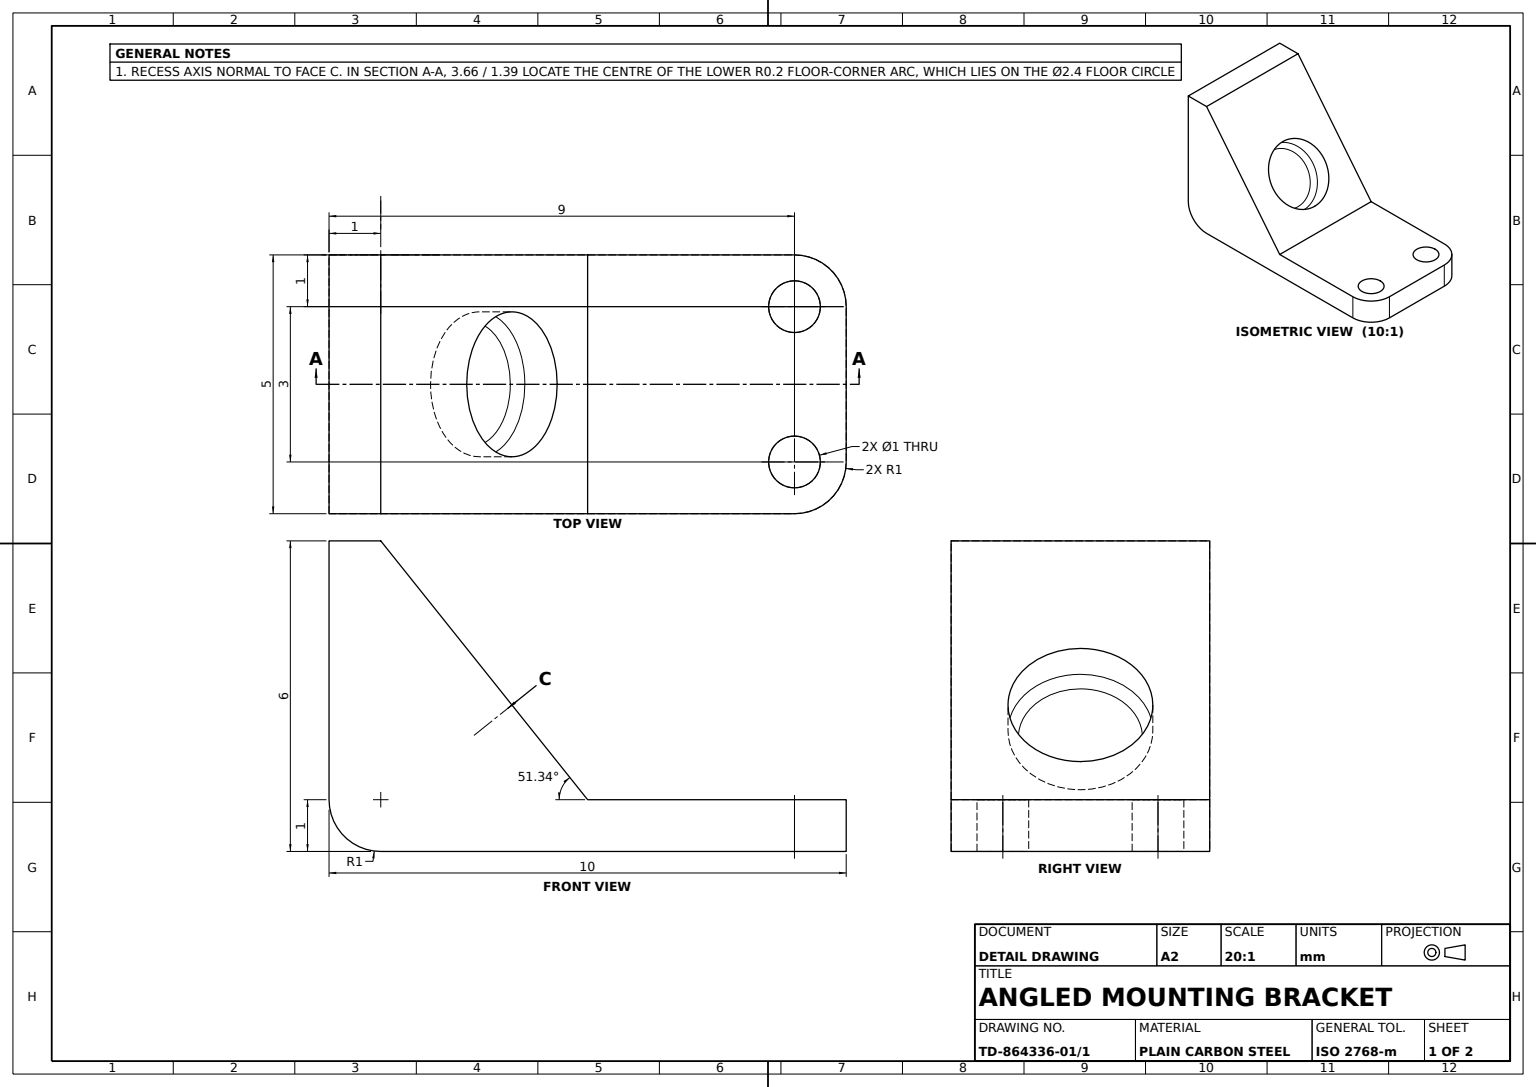
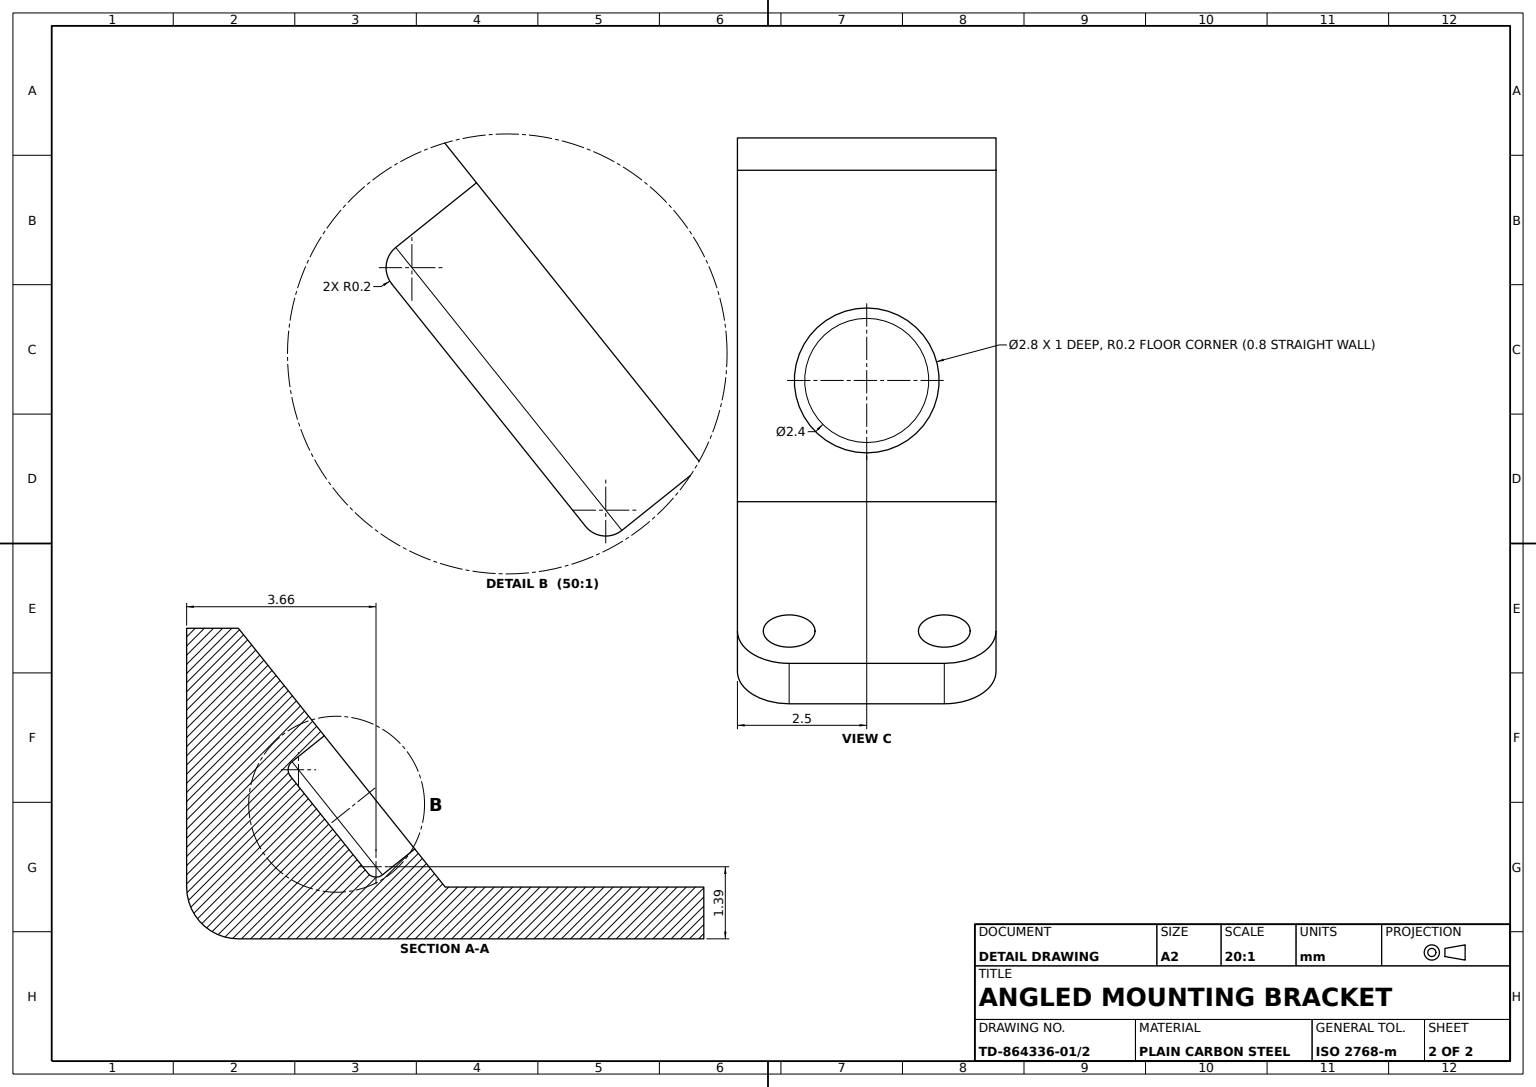
from build123d import *

# Parameters (mm, degrees)
BRACKET_BODY_DEPTH        = 2.5
FACE_RECESS_SKETCH_R      = 1.4
FACE_RECESS_2_8X1_DEPTH   = 1
MOUNTING_HOLES_SKETCH_R   = 0.5
FOOT_MOUNTING_HOLES_DEPTH = 12.456439237
CORNER_FILLETS_R1_R       = 1
RECESS_EDGE_FILLET_R0_2_R = 0.2


with BuildPart() as part:
    # Bracket Profile Sketch → Bracket Body (new, symmetric)
    with BuildSketch(Plane.XY):
        with BuildLine():
            Line((0, 1), (0, 6))
            Line((0, 6), (1, 6))
            Line((1, 6), (5, 1))
            Line((5, 1), (10, 1))
            Line((10, 1), (10, 0))
            Line((10, 0), (1, 0))
            ThreePointArc((1, 0), (0.292893219, 0.292893219), (0, 1))
        make_face()
    extrude(amount=BRACKET_BODY_DEPTH, both=True)

    # Face Recess Sketch → Face Recess Ø2.8x1 (cut)
    with BuildSketch(Plane(origin=(3.536585366, 2.829268293, 0), x_dir=(0, 0, -1), z_dir=(0.7808688094430304, 0.6246950475544242, 0))):
        with Locations(Location((0, 0, 0), (0, 0, 90))):
            Circle(FACE_RECESS_SKETCH_R)
    extrude(amount=-FACE_RECESS_2_8X1_DEPTH, mode=Mode.SUBTRACT)

    # Mounting Holes Sketch → Foot Mounting Holes (cut, through all)
    with BuildSketch(Plane(origin=(0, 1, 0), x_dir=(1, 0, 0), z_dir=(0, 1, 0))):
        with Locations(Location((9, -1.5, 0), (0, 0, 270))):
            Circle(MOUNTING_HOLES_SKETCH_R)
        with Locations(Location((9, 1.5, 0), (0, 0, 270))):
            Circle(MOUNTING_HOLES_SKETCH_R)
    extrude(amount=-FOOT_MOUNTING_HOLES_DEPTH, mode=Mode.SUBTRACT)

    # Corner Fillets R1
    corner_fillets_r1_edges = [part.edges().sort_by_distance(p)[0] for p in [
        (10, 0.5, 2.5),
        (10, 0.5, -2.5),
    ]]
    fillet(corner_fillets_r1_edges, radius=CORNER_FILLETS_R1_R)

    # Recess Edge Fillet R0.2
    recess_edge_fillet_r0_2_edges = [part.edges().sort_by_distance(p)[0] for p in [
        (3.630289623, 1.111356912, 0),
    ]]
    fillet(recess_edge_fillet_r0_2_edges, radius=RECESS_EDGE_FILLET_R0_2_R)


solid = part.part
